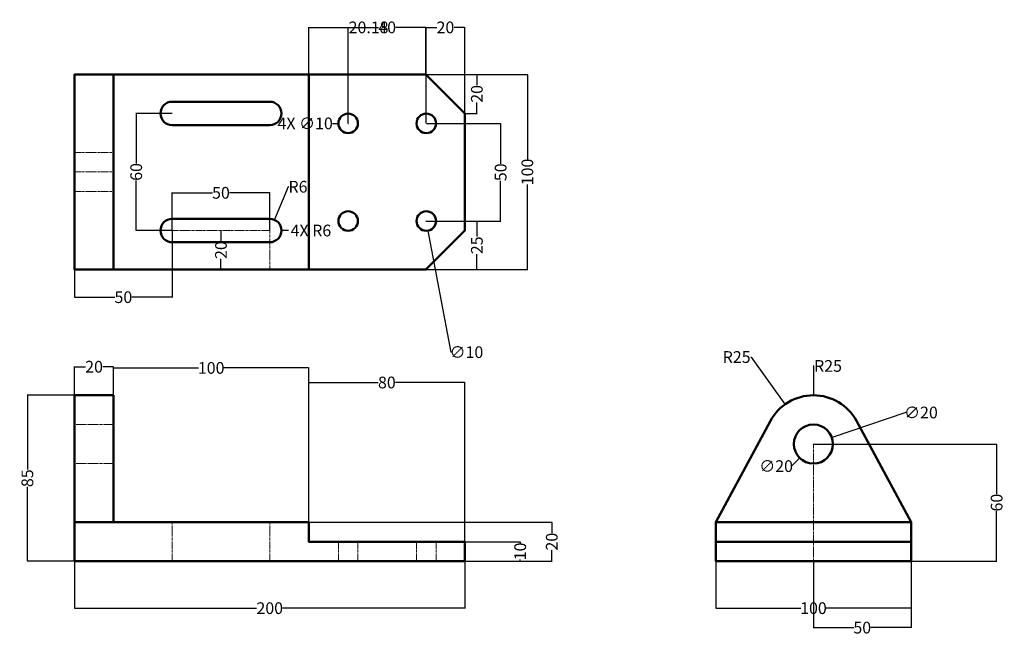
# Model space of a CAD drawing. Units: millimetres. Extents: x 9 to 514, y 122 to 438.
import ezdxf

# ---------------------------------------------------------------- set-up
doc = ezdxf.new("R2010")
doc.units = ezdxf.units.MM
doc.header["$MEASUREMENT"] = 0
doc.linetypes.add('CENTER', pattern=[2, 1.25, -0.25, 0.25, -0.25])
for name, color, linetype, lineweight in [('M-CNTR', 4, 'CENTER', 18), ('M-DIMS', 2, 'Continuous', 25), ('M-OUTL', 7, 'Continuous', 50)]:
    doc.layers.add(name, color=color, linetype=linetype, lineweight=lineweight)
doc.styles.get("Standard").update_dxf_attribs({"font": 'arial.ttf'})
doc.dimstyles.get("Standard").update_dxf_attribs({"dimtxt": 6, "dimasz": 0.18, "dimexe": 0.18, "dimexo": 0.0625, "dimgap": 0.09, "dimtad": 0, "dimtoh": 1, "dimdec": 0, "dimzin": 0, "dimdsep": 46, "dimtxsty": 'Standard', "dimcen": 0.09, "dimadec": 0, "dimazin": 0, "dimtfac": 1, "dimtdec": 0, "dimtofl": 0, "dimtmove": 0, "dimatfit": 3, "dimfxl": 1, "dimtolj": 1, "dimtzin": 0, "dimarcsym": 0})

# ---------------------------------------------------------------- blocks, each defined once
blk = doc.blocks.new('*U1')
at = {"layer": 'M-CNTR', "color": 0, "transparency": 16777216}
blk.add_line((-25.12, 0), (25.12, 0), dxfattribs=at)
blk = doc.blocks.new('*D2')
at = {"layer": 'Defpoints', "color": 0, "transparency": 16777216}
for p in [(425.6, 223.66), (406.68, 217.19)]:
    blk.add_point(p, dxfattribs=at)
at = {"layer": 'M-DIMS', "color": 0, "lineweight": -2, "transparency": 16777216}
for p, q in [((463.39, 236.57), (425.77, 223.71)), ((463.57, 236.57), (463.39, 236.57)), ((416.05, 220.42), (416.23, 220.42)), ((416.14, 220.33), (416.14, 220.51))]:
    blk.add_line(p, q, dxfattribs=at)
at = {"layer": 'M-DIMS', "color": 0, "transparency": 16777216}
blk.add_solid([(425.76, 223.74), (425.78, 223.69), (425.6, 223.66)], dxfattribs=at)
at = {"layer": 'M-DIMS', "color": 0, "transparency": 16777216, "insert": (471.21, 236.57), "char_height": 6, "attachment_point": 5}
blk.add_mtext('\\A1;∅20', dxfattribs=at)
blk = doc.blocks.new('*D3')
at = {"layer": 'Defpoints', "color": 0, "transparency": 16777216}
for p in [(216.85, 339.57), (218.72, 329.75)]:
    blk.add_point(p, dxfattribs=at)
at = {"layer": 'M-DIMS', "color": 0, "lineweight": -2, "transparency": 16777216}
for p, q in [((217.69, 334.66), (217.87, 334.66)), ((217.78, 334.57), (217.78, 334.75)), ((230.54, 267.48), (218.75, 329.57)), ((230.72, 267.48), (230.54, 267.48))]:
    blk.add_line(p, q, dxfattribs=at)
at = {"layer": 'M-DIMS', "color": 0, "transparency": 16777216}
blk.add_solid([(218.78, 329.58), (218.72, 329.57), (218.72, 329.75)], dxfattribs=at)
at = {"layer": 'M-DIMS', "color": 0, "transparency": 16777216, "insert": (238.36, 267.48), "char_height": 6, "attachment_point": 5}
blk.add_mtext('\\A1;∅10', dxfattribs=at)
blk = doc.blocks.new('*D4')
at = {"layer": 'Defpoints', "color": 0, "transparency": 16777216}
for p in [(401.6, 240.76), (416.14, 220.42)]:
    blk.add_point(p, dxfattribs=at)
at = {"layer": 'M-DIMS', "color": 0, "lineweight": -2, "transparency": 16777216}
for p, q in [((384.08, 265), (384.26, 265)), ((384.26, 265), (401.49, 240.9)), ((416.05, 220.42), (416.23, 220.42)), ((416.14, 220.33), (416.14, 220.51))]:
    blk.add_line(p, q, dxfattribs=at)
at = {"layer": 'M-DIMS', "color": 0, "transparency": 16777216}
blk.add_solid([(401.52, 240.92), (401.47, 240.89), (401.6, 240.76)], dxfattribs=at)
at = {"layer": 'M-DIMS', "color": 0, "transparency": 16777216, "insert": (376.8, 265), "char_height": 6, "attachment_point": 5}
blk.add_mtext('\\A1;R25', dxfattribs=at)
blk = doc.blocks.new('*D5')
at = {"layer": 'Defpoints', "color": 0, "transparency": 16777216}
for p in [(416.23, 220.42), (416.14, 160.42), (509.98, 160.42)]:
    blk.add_point(p, dxfattribs=at)
at = {"layer": 'M-DIMS', "color": 0, "lineweight": -2, "transparency": 16777216}
for p, q in [((416.29, 220.42), (510.16, 220.42)), ((509.98, 220.24), (509.98, 194.82)), ((509.98, 160.6), (509.98, 186.03)), ((416.2, 160.42), (510.16, 160.42))]:
    blk.add_line(p, q, dxfattribs=at)
at = {"layer": 'M-DIMS', "color": 0, "transparency": 16777216}
for points in [[(509.95, 220.24), (510.01, 220.24), (509.98, 220.42)], [(509.95, 160.6), (510.01, 160.6), (509.98, 160.42)]]:
    blk.add_solid(points, dxfattribs=at)
at = {"layer": 'M-DIMS', "color": 0, "transparency": 16777216, "insert": (509.98, 190.42), "char_height": 6, "attachment_point": 5, "rotation": 90}
blk.add_mtext('\\A1;60', dxfattribs=at)
blk = doc.blocks.new('*D6')
at = {"layer": 'Defpoints', "color": 0, "transparency": 16777216}
for p in [(416.14, 160.42), (466.14, 160.42), (466.14, 126.4)]:
    blk.add_point(p, dxfattribs=at)
at = {"layer": 'M-DIMS', "color": 0, "lineweight": -2, "transparency": 16777216}
for p, q in [((416.14, 160.36), (416.14, 126.22)), ((466.14, 160.36), (466.14, 126.22)), ((416.32, 126.4), (436.76, 126.4)), ((465.96, 126.4), (445.52, 126.4))]:
    blk.add_line(p, q, dxfattribs=at)
at = {"layer": 'M-DIMS', "color": 0, "transparency": 16777216}
for points in [[(416.32, 126.43), (416.32, 126.37), (416.14, 126.4)], [(465.96, 126.43), (465.96, 126.37), (466.14, 126.4)]]:
    blk.add_solid(points, dxfattribs=at)
at = {"layer": 'M-DIMS', "color": 0, "transparency": 16777216, "insert": (441.14, 126.4), "char_height": 6, "attachment_point": 5}
blk.add_mtext('\\A1;50', dxfattribs=at)
blk = doc.blocks.new('*D7')
at = {"layer": 'Defpoints', "color": 0, "transparency": 16777216}
for p in [(57.6, 260.03), (37.6, 245.42), (57.6, 245.42)]:
    blk.add_point(p, dxfattribs=at)
at = {"layer": 'M-DIMS', "color": 0, "lineweight": -2, "transparency": 16777216}
for p, q in [((37.6, 245.48), (37.6, 260.21)), ((37.78, 260.03), (43.18, 260.03)), ((57.42, 260.03), (52.03, 260.03)), ((57.6, 245.48), (57.6, 260.21))]:
    blk.add_line(p, q, dxfattribs=at)
at = {"layer": 'M-DIMS', "color": 0, "transparency": 16777216}
for points in [[(37.78, 260.06), (37.78, 260), (37.6, 260.03)], [(57.42, 260.06), (57.42, 260), (57.6, 260.03)]]:
    blk.add_solid(points, dxfattribs=at)
at = {"layer": 'M-DIMS', "color": 0, "transparency": 16777216, "insert": (47.6, 260.03), "char_height": 6, "attachment_point": 5}
blk.add_mtext('\\A1;20', dxfattribs=at)
blk = doc.blocks.new('*D8')
at = {"layer": 'Defpoints', "color": 0, "transparency": 16777216}
for p in [(157.6, 259.41), (57.6, 180.42), (157.6, 175.42)]:
    blk.add_point(p, dxfattribs=at)
at = {"layer": 'M-DIMS', "color": 0, "lineweight": -2, "transparency": 16777216}
for p, q in [((57.6, 180.48), (57.6, 259.59)), ((57.78, 259.41), (101.18, 259.41)), ((157.42, 259.41), (114.03, 259.41)), ((157.6, 175.48), (157.6, 259.59))]:
    blk.add_line(p, q, dxfattribs=at)
at = {"layer": 'M-DIMS', "color": 0, "transparency": 16777216}
for points in [[(57.78, 259.44), (57.78, 259.38), (57.6, 259.41)], [(157.42, 259.44), (157.42, 259.38), (157.6, 259.41)]]:
    blk.add_solid(points, dxfattribs=at)
at = {"layer": 'M-DIMS', "color": 0, "transparency": 16777216, "insert": (107.6, 259.41), "char_height": 6, "attachment_point": 5}
blk.add_mtext('\\A1;100', dxfattribs=at)
blk = doc.blocks.new('*D9')
at = {"layer": 'Defpoints', "color": 0, "transparency": 16777216}
for p in [(237.6, 251.95), (157.6, 170.42), (237.6, 170.42)]:
    blk.add_point(p, dxfattribs=at)
at = {"layer": 'M-DIMS', "color": 0, "lineweight": -2, "transparency": 16777216}
for p, q in [((157.6, 170.48), (157.6, 252.13)), ((157.78, 251.95), (193.22, 251.95)), ((237.42, 251.95), (201.99, 251.95)), ((237.6, 170.48), (237.6, 252.13))]:
    blk.add_line(p, q, dxfattribs=at)
at = {"layer": 'M-DIMS', "color": 0, "transparency": 16777216}
for points in [[(157.78, 251.98), (157.78, 251.92), (157.6, 251.95)], [(237.42, 251.98), (237.42, 251.92), (237.6, 251.95)]]:
    blk.add_solid(points, dxfattribs=at)
at = {"layer": 'M-DIMS', "color": 0, "transparency": 16777216, "insert": (197.6, 251.95), "char_height": 6, "attachment_point": 5}
blk.add_mtext('\\A1;80', dxfattribs=at)
blk = doc.blocks.new('*D10')
at = {"layer": 'Defpoints', "color": 0, "transparency": 16777216}
for p in [(237.6, 170.42), (237.6, 160.42), (265.9, 160.42)]:
    blk.add_point(p, dxfattribs=at)
at = {"layer": 'M-DIMS', "color": 0, "lineweight": -2, "transparency": 16777216}
for p, q in [((237.67, 170.42), (266.08, 170.42)), ((265.9, 170.24), (265.9, 169.52)), ((237.67, 160.42), (266.08, 160.42)), ((265.9, 160.6), (265.9, 161.33))]:
    blk.add_line(p, q, dxfattribs=at)
at = {"layer": 'M-DIMS', "color": 0, "transparency": 16777216}
for points in [[(265.87, 170.24), (265.93, 170.24), (265.9, 170.42)], [(265.87, 160.6), (265.93, 160.6), (265.9, 160.42)]]:
    blk.add_solid(points, dxfattribs=at)
at = {"layer": 'M-DIMS', "color": 0, "transparency": 16777216, "insert": (265.9, 165.42), "char_height": 6, "attachment_point": 5, "rotation": 90}
blk.add_mtext('\\A1;10', dxfattribs=at)
blk = doc.blocks.new('*D11')
at = {"layer": 'Defpoints', "color": 0, "transparency": 16777216}
for p in [(157.6, 180.42), (157.6, 160.42), (282.08, 160.42)]:
    blk.add_point(p, dxfattribs=at)
at = {"layer": 'M-DIMS', "color": 0, "lineweight": -2, "transparency": 16777216}
for p, q in [((157.67, 180.42), (282.26, 180.42)), ((282.08, 180.24), (282.08, 174.85)), ((282.08, 160.6), (282.08, 165.99)), ((157.67, 160.42), (282.26, 160.42))]:
    blk.add_line(p, q, dxfattribs=at)
at = {"layer": 'M-DIMS', "color": 0, "transparency": 16777216}
for points in [[(282.05, 180.24), (282.11, 180.24), (282.08, 180.42)], [(282.05, 160.6), (282.11, 160.6), (282.08, 160.42)]]:
    blk.add_solid(points, dxfattribs=at)
at = {"layer": 'M-DIMS', "color": 0, "transparency": 16777216, "insert": (282.08, 170.42), "char_height": 6, "attachment_point": 5, "rotation": 90}
blk.add_mtext('\\A1;20', dxfattribs=at)
blk = doc.blocks.new('*D12')
at = {"layer": 'Defpoints', "color": 0, "transparency": 16777216}
for p in [(137.6, 349.1), (87.6, 329.78), (137.6, 329.78)]:
    blk.add_point(p, dxfattribs=at)
at = {"layer": 'M-DIMS', "color": 0, "lineweight": -2, "transparency": 16777216}
for p, q in [((87.6, 329.84), (87.6, 349.28)), ((87.78, 349.1), (108.23, 349.1)), ((137.42, 349.1), (116.98, 349.1)), ((137.6, 329.84), (137.6, 349.28))]:
    blk.add_line(p, q, dxfattribs=at)
at = {"layer": 'M-DIMS', "color": 0, "transparency": 16777216}
for points in [[(87.78, 349.13), (87.78, 349.07), (87.6, 349.1)], [(137.42, 349.13), (137.42, 349.07), (137.6, 349.1)]]:
    blk.add_solid(points, dxfattribs=at)
at = {"layer": 'M-DIMS', "color": 0, "transparency": 16777216, "insert": (112.6, 349.1), "char_height": 6, "attachment_point": 5}
blk.add_mtext('\\A1;50', dxfattribs=at)
blk = doc.blocks.new('*D13')
at = {"layer": 'Defpoints', "color": 0, "transparency": 16777216}
for p in [(139.92, 335.32), (137.6, 329.78)]:
    blk.add_point(p, dxfattribs=at)
at = {"layer": 'M-DIMS', "color": 0, "lineweight": -2, "transparency": 16777216}
for p, q in [((146.98, 352.2), (139.99, 335.48)), ((147.16, 352.2), (146.98, 352.2)), ((137.51, 329.78), (137.69, 329.78)), ((137.6, 329.69), (137.6, 329.87))]:
    blk.add_line(p, q, dxfattribs=at)
at = {"layer": 'M-DIMS', "color": 0, "transparency": 16777216}
blk.add_solid([(139.96, 335.49), (140.02, 335.47), (139.92, 335.32)], dxfattribs=at)
at = {"layer": 'M-DIMS', "color": 0, "transparency": 16777216, "insert": (152.08, 352.2), "char_height": 6, "attachment_point": 5}
blk.add_mtext('\\A1;R6', dxfattribs=at)
blk = doc.blocks.new('*D14')
at = {"layer": 'Defpoints', "color": 0, "transparency": 16777216}
for p in [(112.6, 329.78), (112.6, 309.78), (112.6, 309.78)]:
    blk.add_point(p, dxfattribs=at)
at = {"layer": 'M-DIMS', "color": 0, "lineweight": -2, "transparency": 16777216}
for p, q in [((112.6, 329.6), (112.6, 324.21)), ((112.67, 329.78), (112.78, 329.78)), ((112.6, 309.96), (112.6, 315.35)), ((112.67, 309.78), (112.78, 309.78))]:
    blk.add_line(p, q, dxfattribs=at)
at = {"layer": 'M-DIMS', "color": 0, "transparency": 16777216}
for points in [[(112.57, 329.6), (112.63, 329.6), (112.6, 329.78)], [(112.57, 309.96), (112.63, 309.96), (112.6, 309.78)]]:
    blk.add_solid(points, dxfattribs=at)
at = {"layer": 'M-DIMS', "color": 0, "transparency": 16777216, "insert": (112.6, 319.78), "char_height": 6, "attachment_point": 5, "rotation": 90}
blk.add_mtext('\\A1;20', dxfattribs=at)
blk = doc.blocks.new('*D15')
at = {"layer": 'Defpoints', "color": 0, "transparency": 16777216}
for p in [(37.6, 329.78), (87.6, 329.78), (37.6, 295.65)]:
    blk.add_point(p, dxfattribs=at)
at = {"layer": 'M-DIMS', "color": 0, "lineweight": -2, "transparency": 16777216}
for p, q in [((37.6, 329.72), (37.6, 295.47)), ((87.6, 329.72), (87.6, 295.47)), ((37.78, 295.65), (58.23, 295.65)), ((87.42, 295.65), (66.98, 295.65))]:
    blk.add_line(p, q, dxfattribs=at)
at = {"layer": 'M-DIMS', "color": 0, "transparency": 16777216}
for points in [[(37.78, 295.68), (37.78, 295.62), (37.6, 295.65)], [(87.42, 295.68), (87.42, 295.62), (87.6, 295.65)]]:
    blk.add_solid(points, dxfattribs=at)
at = {"layer": 'M-DIMS', "color": 0, "transparency": 16777216, "insert": (62.6, 295.65), "char_height": 6, "attachment_point": 5}
blk.add_mtext('\\A1;50', dxfattribs=at)
blk = doc.blocks.new('*D16')
at = {"layer": 'Defpoints', "color": 0, "transparency": 16777216}
for p in [(87.6, 389.78), (69.19, 329.78), (87.48, 329.78)]:
    blk.add_point(p, dxfattribs=at)
at = {"layer": 'M-DIMS', "color": 0, "lineweight": -2, "transparency": 16777216}
for p, q in [((87.54, 389.78), (69.01, 389.78)), ((69.19, 389.6), (69.19, 364.17)), ((69.19, 329.96), (69.19, 355.39)), ((87.42, 329.78), (69.01, 329.78))]:
    blk.add_line(p, q, dxfattribs=at)
at = {"layer": 'M-DIMS', "color": 0, "transparency": 16777216}
for points in [[(69.16, 389.6), (69.22, 389.6), (69.19, 389.78)], [(69.16, 329.96), (69.22, 329.96), (69.19, 329.78)]]:
    blk.add_solid(points, dxfattribs=at)
at = {"layer": 'M-DIMS', "color": 0, "transparency": 16777216, "insert": (69.19, 359.78), "char_height": 6, "attachment_point": 5, "rotation": 90}
blk.add_mtext('\\A1;60', dxfattribs=at)
blk = doc.blocks.new('*D17')
at = {"layer": 'Defpoints', "color": 0, "transparency": 16777216}
for p in [(217.6, 409.78), (217.6, 309.78), (269.58, 309.78)]:
    blk.add_point(p, dxfattribs=at)
at = {"layer": 'M-DIMS', "color": 0, "lineweight": -2, "transparency": 16777216}
for p, q in [((217.67, 409.78), (269.76, 409.78)), ((269.58, 409.6), (269.58, 366.21)), ((269.58, 309.96), (269.58, 353.35)), ((217.67, 309.78), (269.76, 309.78))]:
    blk.add_line(p, q, dxfattribs=at)
at = {"layer": 'M-DIMS', "color": 0, "transparency": 16777216}
for points in [[(269.55, 409.6), (269.61, 409.6), (269.58, 409.78)], [(269.55, 309.96), (269.61, 309.96), (269.58, 309.78)]]:
    blk.add_solid(points, dxfattribs=at)
at = {"layer": 'M-DIMS', "color": 0, "transparency": 16777216, "insert": (269.58, 359.78), "char_height": 6, "attachment_point": 5, "rotation": 90}
blk.add_mtext('\\A1;100', dxfattribs=at)
blk = doc.blocks.new('*D18')
at = {"layer": 'Defpoints', "color": 0, "transparency": 16777216}
for p in [(217.78, 384.66), (217.78, 334.57), (255.89, 334.57)]:
    blk.add_point(p, dxfattribs=at)
at = {"layer": 'M-DIMS', "color": 0, "lineweight": -2, "transparency": 16777216}
for p, q in [((217.85, 384.66), (256.07, 384.66)), ((255.89, 384.48), (255.89, 363.99)), ((255.89, 334.75), (255.89, 355.24)), ((217.85, 334.57), (256.07, 334.57))]:
    blk.add_line(p, q, dxfattribs=at)
at = {"layer": 'M-DIMS', "color": 0, "transparency": 16777216}
for points in [[(255.86, 384.48), (255.92, 384.48), (255.89, 384.66)], [(255.86, 334.75), (255.92, 334.75), (255.89, 334.57)]]:
    blk.add_solid(points, dxfattribs=at)
at = {"layer": 'M-DIMS', "color": 0, "transparency": 16777216, "insert": (255.89, 359.62), "char_height": 6, "attachment_point": 5, "rotation": 90}
blk.add_mtext('\\A1;50', dxfattribs=at)
blk = doc.blocks.new('*D19')
at = {"layer": 'Defpoints', "color": 0, "transparency": 16777216}
for p in [(237.6, 409.78), (243.71, 409.78), (237.6, 389.78)]:
    blk.add_point(p, dxfattribs=at)
at = {"layer": 'M-DIMS', "color": 0, "lineweight": -2, "transparency": 16777216}
for p, q in [((237.67, 409.78), (243.89, 409.78)), ((243.71, 409.6), (243.71, 404.21)), ((243.71, 389.96), (243.71, 395.35)), ((237.67, 389.78), (243.89, 389.78))]:
    blk.add_line(p, q, dxfattribs=at)
at = {"layer": 'M-DIMS', "color": 0, "transparency": 16777216}
for points in [[(243.68, 409.6), (243.74, 409.6), (243.71, 409.78)], [(243.68, 389.96), (243.74, 389.96), (243.71, 389.78)]]:
    blk.add_solid(points, dxfattribs=at)
at = {"layer": 'M-DIMS', "color": 0, "transparency": 16777216, "insert": (243.71, 399.78), "char_height": 6, "attachment_point": 5, "rotation": 90}
blk.add_mtext('\\A1;20', dxfattribs=at)
blk = doc.blocks.new('*D20')
at = {"layer": 'Defpoints', "color": 0, "transparency": 16777216}
for p in [(217.69, 334.66), (217.6, 309.78), (243.71, 309.78)]:
    blk.add_point(p, dxfattribs=at)
at = {"layer": 'M-DIMS', "color": 0, "lineweight": -2, "transparency": 16777216}
for p, q in [((217.76, 334.66), (243.89, 334.66)), ((243.71, 334.48), (243.71, 326.68)), ((243.71, 309.96), (243.71, 317.76)), ((217.67, 309.78), (243.89, 309.78))]:
    blk.add_line(p, q, dxfattribs=at)
at = {"layer": 'M-DIMS', "color": 0, "transparency": 16777216}
for points in [[(243.68, 334.48), (243.74, 334.48), (243.71, 334.66)], [(243.68, 309.96), (243.74, 309.96), (243.71, 309.78)]]:
    blk.add_solid(points, dxfattribs=at)
at = {"layer": 'M-DIMS', "color": 0, "transparency": 16777216, "insert": (243.71, 322.22), "char_height": 6, "attachment_point": 5, "rotation": 90}
blk.add_mtext('\\A1;25', dxfattribs=at)
blk = doc.blocks.new('*D21')
at = {"layer": 'Defpoints', "color": 0, "transparency": 16777216}
for p in [(237.6, 433.83), (217.6, 409.78), (237.6, 389.78)]:
    blk.add_point(p, dxfattribs=at)
at = {"layer": 'M-DIMS', "color": 0, "lineweight": -2, "transparency": 16777216}
for p, q in [((217.6, 409.84), (217.6, 434.01)), ((217.78, 433.83), (223.18, 433.83)), ((237.42, 433.83), (232.03, 433.83)), ((237.6, 389.84), (237.6, 434.01))]:
    blk.add_line(p, q, dxfattribs=at)
at = {"layer": 'M-DIMS', "color": 0, "transparency": 16777216}
for points in [[(217.78, 433.86), (217.78, 433.8), (217.6, 433.83)], [(237.42, 433.86), (237.42, 433.8), (237.6, 433.83)]]:
    blk.add_solid(points, dxfattribs=at)
at = {"layer": 'M-DIMS', "color": 0, "transparency": 16777216, "insert": (227.6, 433.83), "char_height": 6, "attachment_point": 5}
blk.add_mtext('\\A1;20', dxfattribs=at)
blk = doc.blocks.new('*D22')
at = {"layer": 'Defpoints', "color": 0, "transparency": 16777216}
for p in [(217.78, 433.83), (177.78, 384.66), (217.78, 384.66)]:
    blk.add_point(p, dxfattribs=at)
at = {"layer": 'M-DIMS', "color": 0, "lineweight": -2, "transparency": 16777216}
for p, q in [((177.78, 384.72), (177.78, 434.01)), ((177.96, 433.83), (193.29, 433.83)), ((217.6, 433.83), (202.28, 433.83)), ((217.78, 384.72), (217.78, 434.01))]:
    blk.add_line(p, q, dxfattribs=at)
at = {"layer": 'M-DIMS', "color": 0, "transparency": 16777216}
for points in [[(177.96, 433.86), (177.96, 433.8), (177.78, 433.83)], [(217.6, 433.86), (217.6, 433.8), (217.78, 433.83)]]:
    blk.add_solid(points, dxfattribs=at)
at = {"layer": 'M-DIMS', "color": 0, "transparency": 16777216, "insert": (197.78, 433.83), "char_height": 6, "attachment_point": 5}
blk.add_mtext('\\A1;40', dxfattribs=at)
blk = doc.blocks.new('*D23')
at = {"layer": 'Defpoints', "color": 0, "transparency": 16777216}
for p in [(177.78, 433.83), (157.6, 409.78), (177.78, 384.66)]:
    blk.add_point(p, dxfattribs=at)
at = {"layer": 'M-DIMS', "color": 0, "lineweight": -2, "transparency": 16777216}
for p, q in [((157.6, 409.84), (157.6, 434.01)), ((157.78, 433.83), (177.6, 433.83)), ((177.78, 384.72), (177.78, 434.01)), ((177.78, 433.83), (177.96, 433.83))]:
    blk.add_line(p, q, dxfattribs=at)
at = {"layer": 'M-DIMS', "color": 0, "transparency": 16777216}
for points in [[(157.78, 433.86), (157.78, 433.8), (157.6, 433.83)], [(177.6, 433.86), (177.6, 433.8), (177.78, 433.83)]]:
    blk.add_solid(points, dxfattribs=at)
at = {"layer": 'M-DIMS', "color": 0, "transparency": 16777216, "insert": (188.24, 433.83), "char_height": 6, "attachment_point": 5}
blk.add_mtext('\\A1;20.18', dxfattribs=at)
blk = doc.blocks.new('*D24')
at = {"layer": 'Defpoints', "color": 0, "transparency": 16777216}
for p in [(13.43, 245.42), (37.6, 245.42), (37.6, 160.42)]:
    blk.add_point(p, dxfattribs=at)
at = {"layer": 'M-DIMS', "color": 0, "lineweight": -2, "transparency": 16777216}
for p, q in [((37.54, 245.42), (13.25, 245.42)), ((13.43, 245.24), (13.43, 207.34)), ((13.43, 160.6), (13.43, 198.51)), ((37.54, 160.42), (13.25, 160.42))]:
    blk.add_line(p, q, dxfattribs=at)
at = {"layer": 'M-DIMS', "color": 0, "transparency": 16777216}
for points in [[(13.4, 245.24), (13.46, 245.24), (13.43, 245.42)], [(13.4, 160.6), (13.46, 160.6), (13.43, 160.42)]]:
    blk.add_solid(points, dxfattribs=at)
at = {"layer": 'M-DIMS', "color": 0, "transparency": 16777216, "insert": (13.43, 202.92), "char_height": 6, "attachment_point": 5, "rotation": 90}
blk.add_mtext('\\A1;85', dxfattribs=at)
blk = doc.blocks.new('*D25')
at = {"layer": 'Defpoints', "color": 0, "transparency": 16777216}
for p in [(37.6, 160.42), (237.6, 160.42), (237.6, 136.37)]:
    blk.add_point(p, dxfattribs=at)
at = {"layer": 'M-DIMS', "color": 0, "lineweight": -2, "transparency": 16777216}
for p, q in [((37.6, 160.36), (37.6, 136.19)), ((237.6, 160.36), (237.6, 136.19)), ((37.78, 136.37), (130.85, 136.37)), ((237.42, 136.37), (144.36, 136.37))]:
    blk.add_line(p, q, dxfattribs=at)
at = {"layer": 'M-DIMS', "color": 0, "transparency": 16777216}
for points in [[(37.78, 136.4), (37.78, 136.34), (37.6, 136.37)], [(237.42, 136.4), (237.42, 136.34), (237.6, 136.37)]]:
    blk.add_solid(points, dxfattribs=at)
at = {"layer": 'M-DIMS', "color": 0, "transparency": 16777216, "insert": (137.6, 136.37), "char_height": 6, "attachment_point": 5}
blk.add_mtext('\\A1;200', dxfattribs=at)
blk = doc.blocks.new('*D26')
at = {"layer": 'Defpoints', "color": 0, "transparency": 16777216}
for p in [(366.14, 160.42), (466.14, 160.42), (466.14, 136.37)]:
    blk.add_point(p, dxfattribs=at)
at = {"layer": 'M-DIMS', "color": 0, "lineweight": -2, "transparency": 16777216}
for p, q in [((366.14, 160.36), (366.14, 136.19)), ((466.14, 160.36), (466.14, 136.19)), ((366.32, 136.37), (409.72, 136.37)), ((465.96, 136.37), (422.57, 136.37))]:
    blk.add_line(p, q, dxfattribs=at)
at = {"layer": 'M-DIMS', "color": 0, "transparency": 16777216}
for points in [[(366.32, 136.4), (366.32, 136.34), (366.14, 136.37)], [(465.96, 136.4), (465.96, 136.34), (466.14, 136.37)]]:
    blk.add_solid(points, dxfattribs=at)
at = {"layer": 'M-DIMS', "color": 0, "transparency": 16777216, "insert": (416.14, 136.37), "char_height": 6, "attachment_point": 5}
blk.add_mtext('\\A1;100', dxfattribs=at)
blk = doc.blocks.new('*D27')
at = {"layer": 'Defpoints', "color": 0, "transparency": 16777216}
for p in [(137.6, 329.78), (143.6, 329.78)]:
    blk.add_point(p, dxfattribs=at)
at = {"layer": 'M-DIMS', "color": 0, "lineweight": -2, "transparency": 16777216}
for p, q in [((137.51, 329.78), (137.69, 329.78)), ((137.6, 329.69), (137.6, 329.87)), ((147.2, 329.78), (143.78, 329.78))]:
    blk.add_line(p, q, dxfattribs=at)
at = {"layer": 'M-DIMS', "color": 0, "transparency": 16777216}
blk.add_solid([(143.78, 329.81), (143.78, 329.75), (143.6, 329.78)], dxfattribs=at)
at = {"layer": 'M-DIMS', "color": 0, "transparency": 16777216, "insert": (158.7, 329.78), "char_height": 6, "attachment_point": 5}
blk.add_mtext('\\A1;4X R6', dxfattribs=at)
blk = doc.blocks.new('*D28')
at = {"layer": 'Defpoints', "color": 0, "transparency": 16777216}
for p in [(172.78, 384.66), (182.78, 384.66)]:
    blk.add_point(p, dxfattribs=at)
at = {"layer": 'M-DIMS', "color": 0, "lineweight": -2, "transparency": 16777216}
for p, q in [((169.78, 384.66), (172.6, 384.66)), ((177.69, 384.66), (177.87, 384.66)), ((177.78, 384.57), (177.78, 384.75))]:
    blk.add_line(p, q, dxfattribs=at)
at = {"layer": 'M-DIMS', "color": 0, "transparency": 16777216}
blk.add_solid([(172.6, 384.69), (172.6, 384.63), (172.78, 384.66)], dxfattribs=at)
at = {"layer": 'M-DIMS', "color": 0, "transparency": 16777216, "insert": (155.74, 384.66), "char_height": 6, "attachment_point": 5}
blk.add_mtext('\\A1;4X ∅10', dxfattribs=at)
blk = doc.blocks.new('*D29')
at = {"layer": 'Defpoints', "color": 0, "transparency": 16777216}
for p in [(423.21, 227.49), (409.07, 213.35)]:
    blk.add_point(p, dxfattribs=at)
at = {"layer": 'M-DIMS', "color": 0, "lineweight": -2, "transparency": 16777216}
for p, q in [((416.05, 220.42), (416.23, 220.42)), ((416.14, 220.33), (416.14, 220.51)), ((404.83, 209.11), (408.94, 213.22)), ((404.65, 209.11), (404.83, 209.11))]:
    blk.add_line(p, q, dxfattribs=at)
at = {"layer": 'M-DIMS', "color": 0, "transparency": 16777216}
blk.add_solid([(408.92, 213.24), (408.96, 213.2), (409.07, 213.35)], dxfattribs=at)
at = {"layer": 'M-DIMS', "color": 0, "transparency": 16777216, "insert": (397.01, 209.11), "char_height": 6, "attachment_point": 5}
blk.add_mtext('\\A1;∅20', dxfattribs=at)
blk = doc.blocks.new('*D30')
at = {"layer": 'Defpoints', "color": 0, "transparency": 16777216}
for p in [(416.14, 245.42), (416.14, 220.42)]:
    blk.add_point(p, dxfattribs=at)
at = {"layer": 'M-DIMS', "color": 0, "lineweight": -2, "transparency": 16777216}
for p, q in [((416.32, 260.42), (416.14, 260.42)), ((416.14, 260.42), (416.14, 245.6)), ((416.05, 220.42), (416.23, 220.42)), ((416.14, 220.33), (416.14, 220.51))]:
    blk.add_line(p, q, dxfattribs=at)
at = {"layer": 'M-DIMS', "color": 0, "transparency": 16777216}
blk.add_solid([(416.11, 245.6), (416.17, 245.6), (416.14, 245.42)], dxfattribs=at)
at = {"layer": 'M-DIMS', "color": 0, "transparency": 16777216, "insert": (423.6, 260.42), "char_height": 6, "attachment_point": 5}
blk.add_mtext('\\A1;R25', dxfattribs=at)

msp = doc.modelspace()

# ---------------------------------------------------------------- linework, layer by layer
at = {"layer": 'M-CNTR'}
for p, q in [((37.485, 369.781), (57.605, 369.781)), ((37.485, 359.781), (57.605, 359.781)), ((37.485, 349.781), (57.605, 349.781)), ((237.191, 334.661), (237.191, 334.661)), ((237.605, 334.661), (237.785, 334.661)), ((87.605, 309.781), (87.605, 329.781)), ((137.605, 329.781), (137.605, 309.781)), ((57.605, 230.422), (37.605, 230.422)), ((416.142, 160.422), (416.142, 220.422)), ((452.494, 220.422), (452.494, 220.422)), ((57.605, 210.422), (37.605, 210.422)), ((87.605, 180.422), (87.605, 160.422)), ((137.605, 180.422), (137.605, 160.422)), ((172.785, 170.422), (172.785, 160.422)), ((182.785, 170.422), (182.785, 160.422)), ((212.785, 170.422), (212.785, 160.422)), ((222.785, 170.422), (222.785, 160.422))]:
    msp.add_line(p, q, dxfattribs=at)
at = {"layer": 'M-OUTL'}
for p, q in [((57.605, 309.781), (57.605, 409.781)), ((157.605, 309.781), (157.605, 409.781)), ((37.605, 245.422), (57.605, 245.422)), ((37.605, 245.422), (37.605, 180.422)), ((57.605, 245.422), (57.605, 180.422)), ((366.142, 170.422), (466.142, 170.422))]:
    msp.add_line(p, q, dxfattribs=at)
for points in [[(237.605, 389.781), (217.605, 409.781), (37.605, 409.781), (37.605, 309.781), (217.605, 309.781), (237.605, 329.781)], [(157.605, 180.422), (157.605, 170.422), (237.605, 170.422), (237.605, 160.422), (37.605, 160.422), (37.605, 180.422)]]:
    msp.add_lwpolyline(points, close=True, dxfattribs=at)
for points in [[(87.605, 383.781), (137.605, 383.781, 1), (137.605, 395.781), (87.605, 395.781, 1)], [(87.605, 323.781), (137.605, 323.781, 1), (137.605, 335.781), (87.605, 335.781, 1)]]:
    msp.add_lwpolyline(points, format="xyb", close=True, dxfattribs=at)
msp.add_lwpolyline([(366.142, 180.422), (366.142, 160.422), (466.142, 160.422), (466.142, 180.422), (438.141, 232.297, 0.5966087), (394.142, 232.297), (366.142, 180.422), (466.142, 180.422)], format="xyb", dxfattribs=at)
for centre, radius in [((177.785, 384.661), 5), ((217.785, 384.661), 5), ((177.785, 334.661), 5), ((217.785, 334.661), 5), ((416.142, 220.422), 10)]:
    msp.add_circle(centre, radius, dxfattribs=at)

# ---------------------------------------------------------------- block references
at = {"layer": 'M-CNTR'}
msp.add_blockref('*U1', (112.605, 329.781), dxfattribs=at)

# ---------------------------------------------------------------- dimensions: what is measured, and where the dimension line sits
at = {"layer": 'M-DIMS'}
for base, p1, p2, override, picture, middle in [((177.785, 433.831), (157.605, 409.781), (177.785, 384.661), {"dimdec": 2, "dimlfac": 1, "dimrnd": 0, "dimzin": 0, "dimdsep": 46, "dimlunit": 2}, '*D23', (188.236, 433.831)), ((217.785, 433.831), (177.785, 384.661), (217.785, 384.661), {"dimdec": 0, "dimlfac": 1, "dimrnd": 0, "dimzin": 0, "dimdsep": 46, "dimlunit": 2}, '*D22', (197.785, 433.831)), ((237.605, 433.831), (217.605, 409.781), (237.605, 389.781), {"dimdec": 0, "dimlfac": 1, "dimrnd": 0, "dimzin": 0, "dimdsep": 46, "dimlunit": 2}, '*D21', (227.605, 433.831)), ((137.605, 349.097), (87.605, 329.781), (137.605, 329.781), {"dimclrd": 0, "dimclre": 0, "dimclrt": 0}, '*D12', (112.605, 349.097)), ((37.605, 295.648), (87.605, 329.781), (37.605, 329.781), {"dimclrd": 0, "dimclre": 0, "dimclrt": 0}, '*D15', (62.605, 295.648)), ((57.605, 260.027), (37.605, 245.422), (57.605, 245.422), {"dimclrd": 0, "dimclre": 0, "dimclrt": 0}, '*D7', (47.605, 260.027)), ((157.605, 259.406), (57.605, 180.422), (157.605, 175.422), {"dimclrd": 0, "dimclre": 0, "dimclrt": 0}, '*D8', (107.605, 259.406)), ((237.605, 251.948), (157.605, 170.422), (237.605, 170.422), {"dimclrd": 0, "dimclre": 0, "dimclrt": 0}, '*D9', (197.605, 251.948)), ((237.605, 136.372), (37.605, 160.422), (237.605, 160.422), {"dimdec": 0, "dimlfac": 1, "dimrnd": 0, "dimzin": 0, "dimdsep": 46, "dimlunit": 2}, '*D25', (137.605, 136.372)), ((466.142, 136.372), (366.142, 160.422), (466.142, 160.422), {"dimdec": 0, "dimlfac": 1, "dimrnd": 0, "dimzin": 0, "dimdsep": 46, "dimlunit": 2}, '*D26', (416.142, 136.372)), ((466.142, 126.404), (416.142, 160.422), (466.142, 160.422), {"dimclrd": 0, "dimclre": 0, "dimclrt": 0}, '*D6', (441.142, 126.404))]:
    dim = msp.add_linear_dim(base=base, p1=p1, p2=p2, dimstyle='Standard', override=override, dxfattribs=at)
    dim.commit()
    dim.dimension.update_dxf_attribs({"geometry": picture, "text_midpoint": middle})
for base, p1, p2, override, picture, middle in [((269.582, 309.781), (217.605, 409.781), (217.605, 309.781), {"dimclrd": 0, "dimclre": 0, "dimclrt": 0}, '*D17', (269.582, 359.781)), ((243.715, 409.781), (237.605, 389.781), (237.605, 409.781), {"dimclrd": 0, "dimclre": 0, "dimclrt": 0}, '*D19', (243.715, 399.781)), ((69.185, 329.781), (87.605, 389.781), (87.485, 329.781), {"dimclrd": 0, "dimclre": 0, "dimclrt": 0}, '*D16', (69.185, 359.781)), ((255.891, 334.571), (217.785, 384.661), (217.785, 334.571), {"dimclrd": 0, "dimclre": 0, "dimclrt": 0}, '*D18', (255.891, 359.616)), ((243.715, 309.781), (217.695, 334.661), (217.605, 309.781), {"dimclrd": 0, "dimclre": 0, "dimclrt": 0}, '*D20', (243.715, 322.221)), ((112.605, 309.781), (112.605, 329.781), (112.605, 309.781), {"dimclrd": 0, "dimclre": 0, "dimclrt": 0}, '*D14', (112.605, 319.781)), ((13.435, 245.422), (37.605, 160.422), (37.605, 245.422), {"dimdec": 0, "dimlfac": 1, "dimrnd": 0, "dimzin": 0, "dimdsep": 46, "dimlunit": 2}, '*D24', (13.435, 202.922)), ((509.979, 160.422), (416.232, 220.422), (416.142, 160.422), {"dimclrd": 0, "dimclre": 0, "dimclrt": 0}, '*D5', (509.979, 190.422)), ((282.077, 160.422), (157.605, 180.422), (157.605, 160.422), {"dimclrd": 0, "dimclre": 0, "dimclrt": 0}, '*D11', (282.077, 170.422)), ((265.896, 160.422), (237.605, 170.422), (237.605, 160.422), {"dimclrd": 0, "dimclre": 0, "dimclrt": 0}, '*D10', (265.896, 165.422))]:
    dim = msp.add_linear_dim(base=base, p1=p1, p2=p2, angle=90, dimstyle='Standard', override=override, dxfattribs=at)
    dim.commit()
    dim.dimension.update_dxf_attribs({"geometry": picture, "text_midpoint": middle})
dim = msp.add_diameter_dim_2p(p1=(182.785, 384.66), p2=(172.785, 384.661), text='4X <>', dimstyle='Standard', override={"dimdec": 0, "dimlfac": 1, "dimrnd": 0, "dimzin": 0, "dimdsep": 46, "dimlunit": 2}, dxfattribs=at)
dim.commit()
dim.dimension.update_dxf_attribs({"geometry": '*D28', "text_midpoint": (169.785, 384.661), "dimtype": 163})
for center, mpoint, override, picture, middle in [((137.605, 329.781), (139.919, 335.316), {"dimclrd": 0, "dimclre": 0, "dimclrt": 0}, '*D13', (152.085, 352.205)), ((416.142, 220.422), (401.599, 240.757), {"dimclrd": 0, "dimclre": 0, "dimclrt": 0}, '*D4', (376.803, 264.998)), ((416.142, 220.422), (416.142, 245.422), {"dimdec": 0, "dimlfac": 1, "dimrnd": 0, "dimzin": 0, "dimdsep": 46, "dimlunit": 2}, '*D30', (423.603, 260.422))]:
    dim = msp.add_radius_dim(center=center, mpoint=mpoint, dimstyle='Standard', override=override, dxfattribs=at)
    dim.commit()
    dim.dimension.update_dxf_attribs({"geometry": picture, "text_midpoint": middle, "dimtype": 164})
dim = msp.add_radius_dim(center=(137.605, 329.781), mpoint=(143.605, 329.781), text='4X <>', dimstyle='Standard', override={"dimdec": 0, "dimlfac": 1, "dimrnd": 0, "dimzin": 0, "dimdsep": 46, "dimlunit": 2}, dxfattribs=at)
dim.commit()
dim.dimension.update_dxf_attribs({"geometry": '*D27', "text_midpoint": (147.205, 329.781), "dimtype": 164})
for p1, p2, override, picture, middle in [((216.852, 339.573), (218.718, 329.749), {"dimclrd": 0, "dimclre": 0, "dimclrt": 0}, '*D3', (238.364, 267.484)), ((406.679, 217.188), (425.604, 223.656), {"dimclrd": 0, "dimclre": 0, "dimclrt": 0}, '*D2', (471.212, 236.57)), ((423.213, 227.493), (409.071, 213.351), {"dimdec": 0, "dimlfac": 1, "dimrnd": 0, "dimzin": 0, "dimdsep": 46, "dimlunit": 2}, '*D29', (397.007, 209.108))]:
    dim = msp.add_diameter_dim_2p(p1=p1, p2=p2, dimstyle='Standard', override=override, dxfattribs=at)
    dim.commit()
    dim.dimension.update_dxf_attribs({"geometry": picture, "text_midpoint": middle, "dimtype": 163})

doc.saveas('drawing.dxf')
